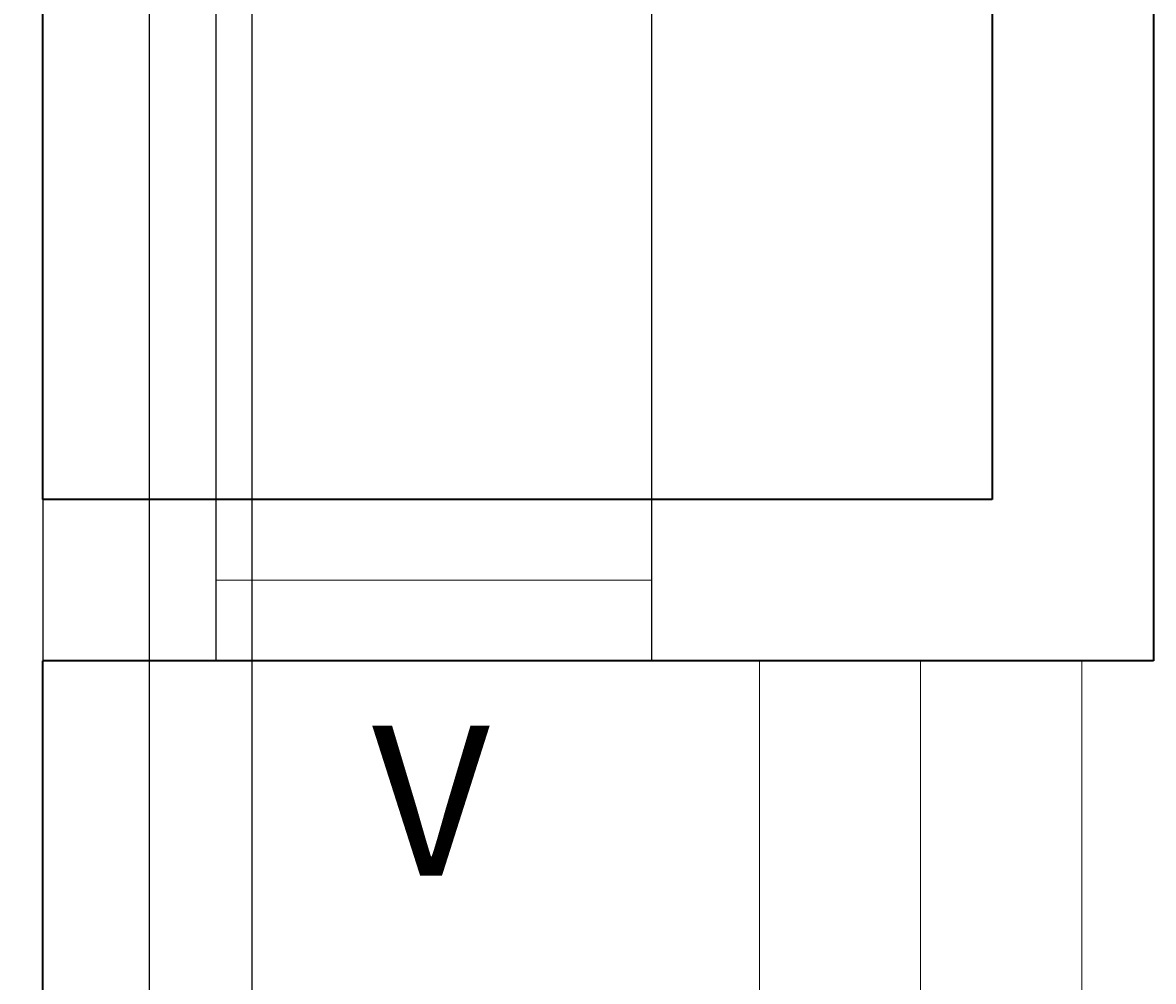
# Model space of a CAD drawing. Units: feet. Extents: x 1654 to 2985, y 1348 to 2230.
# Tile 15 of 53: x 2007 to 2070, y 1643 to 1697. Entities that reach past the tile are written whole.
import ezdxf

# ---------------------------------------------------------------- set-up
doc = ezdxf.new("R2010")
doc.units = ezdxf.units.FT
for name, color, linetype, lineweight in [('A-ANNO-DIMS', 2, 'Continuous', 18), ('A-ANNO-TEXT', 7, 'Continuous', 18), ('A-FLOR-STRS', 7, 'Continuous', 18), ('A-GLAZ', 4, 'Continuous', 18), ('A-WALL', 7, 'Continuous', 35)]:
    doc.layers.add(name, color=color, linetype=linetype, lineweight=lineweight)
doc.styles.get("Standard").update_dxf_attribs({"font": 'arial.ttf'})
doc.dimstyles.get("Standard").update_dxf_attribs({"dimtxt": 0.18, "dimasz": 0.18, "dimexe": 0.18, "dimexo": 0.0625, "dimgap": 0.09, "dimtad": 0, "dimtih": 1, "dimtoh": 1, "dimdec": 4, "dimzin": 0, "dimdsep": 46, "dimtxsty": 'Standard', "dimcen": 0.09, "dimadec": 0, "dimazin": 0, "dimtfac": 1, "dimtdec": 4, "dimtofl": 0, "dimtmove": 0, "dimatfit": 3, "dimfxl": 1, "dimtolj": 1, "dimtzin": 0, "dimarcsym": 0})

# ---------------------------------------------------------------- blocks, each defined once
blk = doc.blocks.new('*D88')
at = {"layer": 'A-ANNO-DIMS', "color": 0, "lineweight": -2, "transparency": 16777216}
for p, q in [((2017.769, 1661.317), (2017.769, 2148.435)), ((2017.949, 2148.255), (2029.547, 2148.255)), ((2041.9, 2148.255), (2030.302, 2148.255)), ((2042.08, 1661.317), (2042.08, 2148.435))]:
    blk.add_line(p, q, dxfattribs=at)
at = {"layer": 'A-ANNO-DIMS', "color": 0, "transparency": 16777216}
for points in [[(2017.949, 2148.285), (2017.949, 2148.225), (2017.769, 2148.255)], [(2041.9, 2148.285), (2041.9, 2148.225), (2042.08, 2148.255)]]:
    blk.add_solid(points, dxfattribs=at)
at = {"layer": 'Defpoints', "color": 0, "transparency": 16777216}
for p in [(2017.769, 2148.255), (2017.769, 1661.255), (2042.08, 1661.255)]:
    blk.add_point(p, dxfattribs=at)
at = {"layer": 'A-ANNO-DIMS', "color": 0, "transparency": 16777216, "insert": (2029.925, 2148.255), "char_height": 0.18, "attachment_point": 5}
blk.add_mtext('\\A1;24.31', dxfattribs=at)
blk = doc.blocks.new('*D101')
at = {"layer": 'A-ANNO-DIMS', "color": 0, "lineweight": -2, "transparency": 16777216}
for p, q in [((1996.092, 2039.192), (1996.092, 1534.075)), ((2014.016, 2039.192), (2014.016, 1534.075)), ((1996.272, 1534.255), (2004.599, 1534.255)), ((2013.836, 1534.255), (2005.509, 1534.255))]:
    blk.add_line(p, q, dxfattribs=at)
at = {"layer": 'A-ANNO-DIMS', "color": 0, "transparency": 16777216}
for points in [[(1996.272, 1534.285), (1996.272, 1534.225), (1996.092, 1534.255)], [(2013.836, 1534.285), (2013.836, 1534.225), (2014.016, 1534.255)]]:
    blk.add_solid(points, dxfattribs=at)
at = {"layer": 'Defpoints', "color": 0, "transparency": 16777216}
for p in [(1996.092, 2039.255), (2014.016, 2039.255), (2014.016, 1534.255)]:
    blk.add_point(p, dxfattribs=at)
at = {"layer": 'A-ANNO-DIMS', "color": 0, "transparency": 16777216, "insert": (2005.054, 1534.255), "char_height": 0.18, "attachment_point": 5}
blk.add_mtext('\\A1;17.924', dxfattribs=at)
blk = doc.blocks.new('*D102')
at = {"layer": 'A-ANNO-DIMS', "color": 0, "lineweight": -2, "transparency": 16777216}
for p, q in [((2008.092, 1742.192), (2008.092, 1534.075)), ((2019.757, 1742.192), (2019.757, 1534.075)), ((2008.272, 1534.255), (2013.47, 1534.255)), ((2019.577, 1534.255), (2014.379, 1534.255))]:
    blk.add_line(p, q, dxfattribs=at)
at = {"layer": 'A-ANNO-DIMS', "color": 0, "transparency": 16777216}
for points in [[(2008.272, 1534.285), (2008.272, 1534.225), (2008.092, 1534.255)], [(2019.577, 1534.285), (2019.577, 1534.225), (2019.757, 1534.255)]]:
    blk.add_solid(points, dxfattribs=at)
at = {"layer": 'Defpoints', "color": 0, "transparency": 16777216}
for p in [(2008.092, 1742.255), (2019.757, 1742.255), (2019.757, 1534.255)]:
    blk.add_point(p, dxfattribs=at)
at = {"layer": 'A-ANNO-DIMS', "color": 0, "transparency": 16777216, "insert": (2013.925, 1534.255), "char_height": 0.18, "attachment_point": 5}
blk.add_mtext('\\A1;11.664', dxfattribs=at)

msp = doc.modelspace()

# ---------------------------------------------------------------- linework, layer by layer
at = {"layer": 'A-FLOR-STRS'}
for p, q in [((2048.0924, 1565.2549), (2048.0924, 1661.2549)), ((2057.0924, 1565.2549), (2057.0924, 1661.2549)), ((2066.0924, 1565.2549), (2066.0924, 1661.2549))]:
    msp.add_line(p, q, dxfattribs=at)
at = {"layer": 'A-GLAZ'}
for p, q in [((2017.7694, 1670.2549), (2017.7694, 1661.2549)), ((2042.0798, 1670.2549), (2042.0798, 1661.2549)), ((2017.7694, 1665.7549), (2042.0798, 1665.7549))]:
    msp.add_line(p, q, dxfattribs=at)
at = {"layer": 'A-WALL'}
for p, q in [((2008.0924, 1670.2549), (2008.0924, 1742.2549)), ((2061.0924, 1742.2549), (2061.0924, 1670.2549)), ((2070.0924, 1742.2549), (2070.0924, 1661.2549)), ((2061.0924, 1670.2549), (2008.0924, 1670.2549)), ((2070.0924, 1661.2549), (2008.0924, 1661.2549)), ((2008.0924, 1600.2549), (2008.0924, 1661.2549))]:
    msp.add_line(p, q, dxfattribs=at)

# ---------------------------------------------------------------- texts
at = {"layer": 'A-ANNO-TEXT'}
msp.add_text('V', height=8.3811, dxfattribs=at).set_placement((2026.4617, 1649.2565))

# ---------------------------------------------------------------- dimensions: what is measured, and where the dimension line sits
at = {"layer": 'A-ANNO-DIMS'}
for base, p1, p2, override, picture, middle in [((2017.7694, 2148.2549), (2042.0798, 1661.2549), (2017.7694, 1661.2549), {"dimdec": 2, "dimlfac": 1, "dimrnd": 0, "dimzin": 0, "dimdsep": 46, "dimlunit": 2}, '*D88', (2029.9246, 2148.2549)), ((2014.016, 1534.2549), (1996.0924, 2039.2549), (2014.016, 2039.2549), {"dimdec": 3, "dimlfac": 1, "dimrnd": 0, "dimzin": 0, "dimdsep": 46, "dimlunit": 2}, '*D101', (2005.0542, 1534.2549)), ((2019.7567, 1534.2549), (2008.0924, 1742.2549), (2019.7567, 1742.2549), {"dimdec": 3, "dimlfac": 1, "dimrnd": 0, "dimzin": 0, "dimdsep": 46, "dimlunit": 2}, '*D102', (2013.9246, 1534.2549))]:
    dim = msp.add_linear_dim(base=base, p1=p1, p2=p2, dimstyle='Standard', override=override, dxfattribs=at)
    dim.commit()
    dim.dimension.update_dxf_attribs({"geometry": picture, "text_midpoint": middle})

doc.saveas('drawing.dxf')
